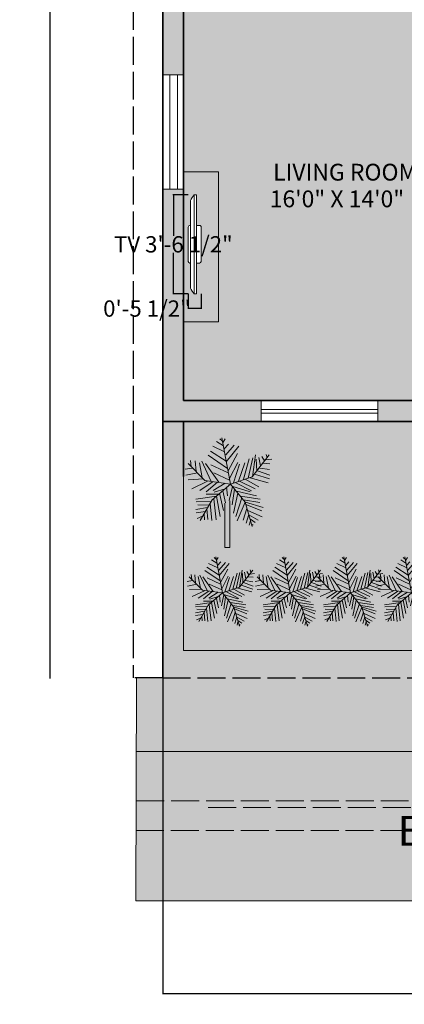
# Model space of a CAD drawing. Units: inches. Extents: x 1316 to 1777, y 813 to 1650.
# Tile 1 of 22: x 1316 to 1481, y 813 to 1237. Entities that reach past the tile are written whole.
import ezdxf

# ---------------------------------------------------------------- set-up
doc = ezdxf.new("R2010")
doc.units = ezdxf.units.IN
doc.header["$MEASUREMENT"] = 0
doc.linetypes.add('ACAD_ISO02W100', pattern=[15, 12, -3])
for name, color, linetype, lineweight in [('A-ANNO-DIMS', 2, 'Continuous', 18), ('A-AREA-IDEN', 7, 'Continuous', 18), ('A-EQPM', 8, 'Continuous', 18), ('A-FURN-PATT', 23, 'Continuous', 13), ('A-WALL-PATT', 250, 'Continuous', 13), ('C-PROP', 8, 'ACAD_ISO02W100', 25), ('C-ROAD', 8, 'Continuous', 18), ('C-ROAD-MARK', 9, 'ACAD_ISO02W100', 13), ('C-ROAD-PATT', 251, 'Continuous', 13), ('furniture', 23, 'Continuous', 18), ('greenary', 106, 'Continuous', 13), ('L-HRDS', 8, 'Continuous', 18), ('L-HRDS-PATT', 252, 'Continuous', 13), ('L-PLNT-PATT', 74, 'Continuous', 13), ('text', 7, 'Continuous', 18), ('walls', 250, 'Continuous', 35), ('windows', 141, 'Continuous', 18)]:
    doc.layers.add(name, color=color, linetype=linetype, lineweight=lineweight)
doc.layers.add('A-FLOR-PATT', color=254, linetype='Continuous', lineweight=13, true_color=0xfeeab9)
doc.styles.get("Standard").update_dxf_attribs({"font": 'arial.ttf'})
doc.dimstyles.get("Standard").update_dxf_attribs({"dimtxt": 7, "dimasz": 0.18, "dimexe": 0.18, "dimexo": 0.0625, "dimgap": 0.09, "dimtad": 0, "dimtih": 1, "dimtoh": 1, "dimzin": 0, "dimdsep": 46, "dimlunit": 3, "dimtxsty": 'Standard', "dimcen": 0.09, "dimadec": 0, "dimazin": 0, "dimtfac": 1, "dimtofl": 0, "dimtmove": 0, "dimatfit": 3, "dimfxl": 1, "dimtolj": 1, "dimtzin": 0, "dimarcsym": 0})

# ---------------------------------------------------------------- blocks, each defined once
blk = doc.blocks.new('PLASMA-LARGE')
at = {"layer": 'furniture'}
for p, q in [((-7.26, 0), (7.26, 0)), ((-21, -2.5), (21, -2.5)), ((-21, -2.5), (-21, -3.5)), ((-21, -3.5), (21, -3.5)), ((-18.61, -1), (18.61, -1)), ((-8, -1), (-8, -0.74)), ((-8, -3.5), (-8, -4.76)), ((8, -1), (8, -0.74)), ((8, -3.5), (8, -4.76)), ((21, -2.5), (21, -3.5)), ((-7.26, -5.5), (7.26, -5.5))]:
    blk.add_line(p, q, dxfattribs=at)
for centre, radius, start, end in [((-7.26, -0.74), 0.744, 90, 180), ((7.26, -0.74), 0.744, 0, 90), ((-13.97, -11.05), 11.07, 114.7602, 129.4175), ((13.97, -11.05), 11.07, 50.5825, 65.2398), ((-7.26, -4.76), 0.744, 180, 270), ((7.26, -4.76), 0.744, 270, 0)]:
    blk.add_arc(centre, radius, start, end, dxfattribs=at)
blk = doc.blocks.new('*U13')
for p, q in [((-8.737, 47.138), (-17.069, 52.711)), ((-10.186, 53.64), (-13.084, 55.962)), ((0, 0), (-10.5, 57)), ((-9.099, 51.782), (-6.563, 55.962)), ((-7.65, 43.423), (-2.578, 49.46)), ((-5.114, 28.097), (-24.676, 40.636)), ((-7.288, 39.707), (-21.778, 46.673)), ((-5.839, 35.992), (4.667, 48.067)), ((-5.114, 27.632), (10.463, 46.673)), ((-2.941, 16.486), (8.652, 37.85)), ((-31.5, 4.5), (-52.5, 25.5)), ((-48.585, 21.131), (-49.309, 29.026)), ((-43.513, 28.561), (-42.427, 15.558)), ((-38.442, 26.239), (-34.819, 7.663)), ((-35.544, 28.097), (-24.314, 3.947)), ((-14.533, 2.09), (-30.834, 25.31)), ((-3.665, 19.273), (-27.574, 35.527)), ((-1.129, 6.734), (9.014, 26.704)), ((3.942, 1.625), (11.187, 24.381)), ((10.101, 3.483), (17.708, 26.239)), ((16.259, 5.805), (23.142, 31.348)), ((22.055, 7.198), (27.489, 32.277)), ((27, 9), (48, 36)), ((27.127, 9.056), (31.112, 35.992)), ((31.836, 30.883), (32.561, 16.486)), ((35.096, 32.741), (37.27, 22.524)), ((38.719, 34.134), (41.979, 28.561)), ((40.53, 25.775), (48.862, 24.846)), ((43.791, 29.954), (51.036, 30.883)), ((44.153, 36.456), (45.239, 32.741)), ((-47.498, 19.737), (-55.83, 18.344)), ((-40.615, 13.7), (-55.105, 10.913)), ((-24.314, 23.917), (-2.941, 13.7)), ((-20.691, 13.7), (-1.129, 4.876)), ((29.662, 12.307), (48.137, 6.269)), ((33.285, 16.486), (48.862, 10.913)), ((36.183, 19.737), (48.137, 17.88)), ((-33.37, 6.269), (-52.207, 5.34)), ((-28.299, 3.483), (-47.86, -5.805)), ((-21.416, 3.018), (-38.079, -8.128)), ((0, 0), (-31.5, 4.5)), ((-15.982, 2.09), (-30.11, -9.521)), ((0, 0), (-22.5, -19.5)), ((-6.563, 1.161), (-21.416, -8.128)), ((0, 0), (27, 9)), ((0, 0), (18, -22.5)), ((6.478, 1.625), (26.04, -8.592)), ((11.187, 3.483), (30.749, -5.805)), ((18.07, 5.805), (35.096, -3.483)), ((24.229, 7.663), (46.688, 1.625)), ((-6.563, -5.805), (-19.967, -9.985)), ((-13.446, -11.378), (-8.737, -32.741)), ((-9.461, -8.592), (-6.201, -23.453)), ((-4.752, -3.483), (-3.665, -14.629)), ((2.493, -3.019), (-1.491, -20.202)), ((1.769, -2.555), (24.229, -9.521)), ((5.029, -6.27), (2.131, -25.775)), ((9.014, -11.378), (3.58, -35.992)), ((7.565, -9.056), (32.198, -14.629)), ((-17.431, -15.094), (-42.789, -18.809)), ((-24.314, -21.596), (-42.427, -22.06)), ((-22.5, -19.5), (-37.5, -45)), ((-15.257, -12.772), (-30.11, -12.772)), ((-25.038, -23.918), (-22.865, -45.281)), ((-20.691, -18.345), (-17.793, -44.352)), ((-17.069, -15.094), (-12.721, -40.172)), ((14.085, -16.951), (6.478, -40.172)), ((18.07, -22.524), (8.289, -45.745)), ((12.274, -15.094), (36.907, -18.809)), ((16.259, -19.738), (36.183, -22.989)), ((18, -22.5), (27, -52.5)), ((18.433, -22.524), (40.53, -29.026)), ((-28.299, -29.026), (-42.789, -31.348)), ((-30.834, -34.135), (-42.427, -35.528)), ((-26.849, -26.24), (-40.253, -25.775)), ((-29.023, -30.884), (-27.936, -43.887)), ((20.244, -30.419), (15.897, -44.816)), ((19.157, -25.311), (38.719, -33.206)), ((21.331, -32.741), (39.081, -40.636)), ((-34.457, -39.708), (-40.978, -42.494)), ((-32.646, -36.921), (-31.921, -44.352)), ((22.78, -37.85), (19.519, -48.532)), ((22.78, -38.314), (34.372, -44.816)), ((24.591, -45.745), (23.142, -50.854)), ((24.591, -43.423), (30.749, -47.603)), ((26.764, -49.925), (28.213, -50.854))]:
    blk.add_line(p, q)
blk = doc.blocks.new('*D23')
at = {"layer": 'A-ANNO-DIMS', "color": 0, "lineweight": -2, "transparency": 16777216}
for p, q in [((1328.47, 1604.17), (1328.87, 1604.17)), ((1328.69, 1603.99), (1328.69, 1282.59)), ((1328.69, 953.87), (1328.69, 1275.27)), ((1328.47, 953.69), (1328.87, 953.69))]:
    blk.add_line(p, q, dxfattribs=at)
at = {"layer": 'A-ANNO-DIMS', "color": 0, "transparency": 16777216}
for points in [[(1328.66, 1603.99), (1328.72, 1603.99), (1328.69, 1604.17)], [(1328.66, 953.87), (1328.72, 953.87), (1328.69, 953.69)]]:
    blk.add_solid(points, dxfattribs=at)
at = {"layer": 'Defpoints', "color": 0, "transparency": 16777216}
for p in [(1328.4, 1604.17), (1328.4, 953.69), (1328.69, 953.69)]:
    blk.add_point(p, dxfattribs=at)
at = {"layer": 'A-ANNO-DIMS', "color": 0, "transparency": 16777216, "insert": (1328.69, 1278.93), "char_height": 7, "width": 24.3281, "attachment_point": 5}
blk.add_mtext('\\A1;47\'-0"', dxfattribs=at)
blk = doc.blocks.new('*D46')
at = {"layer": 'A-ANNO-DIMS', "color": 0, "lineweight": -2, "transparency": 16777216}
for p, q in [((1387.95, 1161.24), (1381.46, 1161.24)), ((1381.64, 1161.06), (1381.64, 1143.71)), ((1381.64, 1118.95), (1381.64, 1136.29)), ((1387.95, 1118.77), (1381.46, 1118.77))]:
    blk.add_line(p, q, dxfattribs=at)
at = {"layer": 'A-ANNO-DIMS', "color": 0, "transparency": 16777216}
for points in [[(1381.61, 1161.06), (1381.67, 1161.06), (1381.64, 1161.24)], [(1381.61, 1118.95), (1381.67, 1118.95), (1381.64, 1118.77)]]:
    blk.add_solid(points, dxfattribs=at)
at = {"layer": 'Defpoints', "color": 0, "transparency": 16777216}
for p in [(1381.64, 1161.24), (1388.01, 1161.24), (1388.01, 1118.77)]:
    blk.add_point(p, dxfattribs=at)
at = {"layer": 'A-ANNO-DIMS', "color": 0, "transparency": 16777216, "insert": (1381.64, 1140), "char_height": 7, "attachment_point": 5}
blk.add_mtext('\\A1;TV 3\'-6 1/2"', dxfattribs=at)
blk = doc.blocks.new('*D47')
at = {"layer": 'A-ANNO-DIMS', "color": 0, "lineweight": -2, "transparency": 16777216}
for p, q in [((1388.01, 1118.7), (1388.01, 1112.21)), ((1393.58, 1118.7), (1393.58, 1112.21)), ((1388.01, 1112.39), (1387.83, 1112.39)), ((1393.4, 1112.39), (1388.19, 1112.39))]:
    blk.add_line(p, q, dxfattribs=at)
at = {"layer": 'A-ANNO-DIMS', "color": 0, "transparency": 16777216}
for points in [[(1388.19, 1112.42), (1388.19, 1112.36), (1388.01, 1112.39)], [(1393.4, 1112.42), (1393.4, 1112.36), (1393.58, 1112.39)]]:
    blk.add_solid(points, dxfattribs=at)
at = {"layer": 'Defpoints', "color": 0, "transparency": 16777216}
for p in [(1388.01, 1118.77), (1393.58, 1118.77), (1388.01, 1112.39)]:
    blk.add_point(p, dxfattribs=at)
at = {"layer": 'A-ANNO-DIMS', "color": 0, "transparency": 16777216, "insert": (1370.29, 1112.39), "char_height": 7, "attachment_point": 5}
blk.add_mtext('\\A1;0\'-5 1/2"', dxfattribs=at)
blk = doc.blocks.new('*D50')
at = {"layer": 'A-ANNO-DIMS', "color": 0, "lineweight": -2, "transparency": 16777216}
for p, q in [((1377.06, 1063.81), (1377.06, 817.77)), ((1713.17, 1031.11), (1713.17, 817.77)), ((1377.24, 817.95), (1532.95, 817.95)), ((1712.99, 817.95), (1557.29, 817.95))]:
    blk.add_line(p, q, dxfattribs=at)
at = {"layer": 'A-ANNO-DIMS', "color": 0, "transparency": 16777216}
for points in [[(1377.24, 817.98), (1377.24, 817.92), (1377.06, 817.95)], [(1712.99, 817.98), (1712.99, 817.92), (1713.17, 817.95)]]:
    blk.add_solid(points, dxfattribs=at)
at = {"layer": 'Defpoints', "color": 0, "transparency": 16777216}
for p in [(1377.06, 1063.87), (1713.17, 1031.17), (1713.17, 817.95)]:
    blk.add_point(p, dxfattribs=at)
at = {"layer": 'A-ANNO-DIMS', "color": 0, "transparency": 16777216, "insert": (1545.12, 817.95), "char_height": 7, "attachment_point": 5}
blk.add_mtext('\\A1;28\'-0"', dxfattribs=at)

msp = doc.modelspace()

# ---------------------------------------------------------------- hatches: boundary and pattern name
at = {"layer": 'A-FLOR-PATT'}
h = msp.add_hatch(color=256, dxfattribs=at)
h.dxf.hatch_style = 1
h.paths.add_polyline_path([(1567.673, 1281.369), (1651.673, 1281.369), (1651.673, 1365.369), (1597.673, 1365.369), (1597.673, 1429.869), (1570.345, 1429.869), (1570.345, 1471.869), (1510.345, 1471.869), (1510.345, 1429.869), (1444.564, 1429.869), (1444.564, 1322.882), (1444.564, 1300.088), (1510.564, 1300.088), (1510.564, 1295.094), (1510.564, 1240.869), (1386.064, 1240.869), (1386.064, 1171.185), (1400.961, 1171.185), (1400.961, 1106.742), (1386.064, 1106.742), (1386.064, 1072.869), (1510.564, 1072.869), (1510.564, 1040.173), (1541.068, 1040.173, -0.367085), (1572.764, 1069.547), (1572.764, 1069.579), (1574.225, 1069.579), (1574.225, 1040.173), (1616.037, 1040.173), (1616.037, 1086.627), (1616.037, 1103.705), (1613.066, 1105.235), (1616.037, 1106.686), (1616.037, 1123.869), (1567.673, 1123.869)])
h.paths.add_polyline_path([(1508.987, 1198.018), (1511.117, 1198.018), (1511.117, 1200.148), (1532.595, 1200.148), (1532.595, 1198.018), (1534.725, 1198.018), (1534.725, 1176.008), (1530.465, 1176.008), (1530.465, 1176.718), (1513.247, 1176.718), (1513.247, 1176.008), (1508.987, 1176.008)], flags=16)
h.paths.add_polyline_path([(1505.979, 1151.315), (1521.504, 1151.315), (1521.504, 1123.623), (1505.979, 1123.623)], flags=16)
h.paths.add_polyline_path([(1507.734, 1150.101, -1), (1506.932, 1150.101, -1)], flags=0)
h.paths.add_polyline_path([(1512.288, 1138.353), (1512.28, 1138.392), (1512.219, 1138.376)], flags=0)
h.paths.add_polyline_path([(1511.539, 1138.926), (1511.802, 1138.967), (1511.817, 1139.27), (1511.607, 1139.246)], flags=0)
h.paths.add_polyline_path([(1513.745, 1140.234), (1513.68, 1139.885), (1514.014, 1140.045), (1513.855, 1140.308)], flags=0)
h.paths.add_polyline_path([(1513.759, 1139.089), (1514.005, 1139.255), (1513.807, 1139.483), (1513.564, 1139.327)], flags=0)
h.paths.add_polyline_path([(1514.219, 1138.385), (1514.336, 1138.33), (1514.544, 1138.32), (1514.802, 1138.874), (1514.451, 1138.716)], flags=0)
h.paths.add_polyline_path([(1514.577, 1137.439), (1514.573, 1137.4), (1514.699, 1137.4), (1514.696, 1137.402)], flags=0)
h.paths.add_polyline_path([(1512.26, 1136.199), (1512.199, 1136.399), (1512.032, 1136.325), (1512.095, 1136.101), (1512.257, 1136.192)], flags=0)
h.paths.add_polyline_path([(1512.644, 1137.274), (1512.356, 1137.23), (1512.432, 1137.049), (1512.703, 1137.093)], flags=0)
h.paths.add_polyline_path([(1513.049, 1137.593), (1512.979, 1137.8), (1512.843, 1137.757), (1512.887, 1137.556)], flags=0)
h.paths.add_polyline_path([(1513.269, 1138.556), (1513.571, 1137.962), (1513.459, 1136.814), (1513.212, 1137.878), (1513.032, 1138.443)], flags=0)
h.paths.add_polyline_path([(1514.891, 1136.377), (1514.696, 1136.401), (1514.683, 1136.246), (1514.87, 1136.165)], flags=0)
h.paths.add_polyline_path([(1514.142, 1137.293), (1514.047, 1136.743), (1514.27, 1136.751), (1514.328, 1137.265)], flags=0)
h.paths.add_polyline_path([(1515.362, 1138.976), (1515.334, 1138.638), (1515.596, 1138.588), (1515.627, 1138.932)], flags=0)
h.paths.add_polyline_path([(1537.285, 1177.912), (1537.995, 1177.912), (1537.995, 1195.13), (1537.285, 1195.13), (1537.285, 1199.39), (1559.295, 1199.39), (1559.295, 1197.26), (1561.425, 1197.26), (1561.425, 1175.782), (1559.295, 1175.782), (1559.295, 1173.652), (1559.379, 1173.652), (1559.379, 1171.514), (1561.517, 1171.514), (1561.517, 1098.819), (1559.379, 1098.819), (1559.379, 1096.68), (1537.285, 1096.68), (1537.285, 1100.957), (1537.997, 1100.957), (1537.997, 1169.376), (1537.285, 1169.376), (1537.285, 1173.652)], flags=16)
h.paths.add_polyline_path([(1518.623, 1345.565), (1519.133, 1345.48), (1519.133, 1345.485), (1518.623, 1345.567)], flags=16)
h.paths.add_polyline_path([(1518.798, 1374.15), (1519.308, 1374.064), (1519.308, 1374.069), (1518.798, 1374.152)], flags=16)
h.paths.add_polyline_path([(1537.764, 1413.501), (1537.678, 1412.991), (1537.683, 1412.991), (1537.766, 1413.501)], flags=16)
h.paths.add_polyline_path([(1572.905, 1373.821), (1573.927, 1373.975), (1574.027, 1390.309), (1573.007, 1390.475), (1573.007, 1390.475)], flags=16)
h.paths.add_polyline_path([(1572.73, 1345.237), (1573.752, 1345.39), (1573.852, 1361.724), (1572.832, 1361.89), (1572.832, 1361.89)], flags=16)
h.paths.add_polyline_path([(1537.211, 1322.643), (1537.364, 1321.621), (1553.698, 1321.521), (1553.864, 1322.541)], flags=16)
h.paths.add_polyline_path([(1535.908, 1331.328), (1527.214, 1331.382), (1527.664, 1404.885), (1564.416, 1404.66), (1563.966, 1331.157), (1555.273, 1331.21), (1553.947, 1323.051), (1537.134, 1323.154)], flags=16)
h.paths.add_polyline_path([(1536.15, 1336.503), (1536.235, 1337.572), (1536.323, 1338.628), (1536.411, 1339.663), (1536.495, 1340.67), (1536.574, 1341.66), (1536.648, 1342.648), (1536.717, 1343.649), (1536.78, 1344.678), (1536.837, 1345.75), (1536.913, 1347.475), (1536.93, 1348.082), (1536.867, 1346.314), (1536.754, 1344.188), (1536.619, 1342.219), (1536.495, 1340.67), (1536.411, 1339.663), (1536.323, 1338.628), (1536.235, 1337.572), (1536.15, 1336.503), (1536.071, 1335.432), (1536.002, 1334.37), (1535.917, 1332.754), (1535.909, 1332.308), (1535.964, 1333.78), (1536.071, 1335.432)], flags=0)
h.paths.add_polyline_path([(1540.412, 1338.345), (1540.539, 1339.037), (1540.667, 1339.758), (1540.798, 1340.518), (1540.93, 1341.325), (1541.063, 1342.187), (1541.196, 1343.109), (1541.326, 1344.085), (1541.45, 1345.102), (1541.566, 1346.15), (1541.669, 1347.219), (1541.758, 1348.296), (1541.829, 1349.371), (1541.879, 1350.434), (1541.906, 1351.476), (1541.91, 1352.5), (1541.895, 1353.512), (1541.861, 1354.518), (1541.812, 1355.524), (1541.749, 1356.537), (1541.674, 1357.561), (1541.551, 1359.062), (1541.495, 1359.67), (1541.589, 1358.603), (1541.721, 1356.977), (1541.846, 1354.98), (1541.912, 1352.982), (1541.903, 1350.951), (1541.806, 1348.87), (1541.628, 1346.713), (1541.396, 1344.612), (1541.135, 1342.656), (1540.872, 1340.947), (1540.617, 1339.466), (1540.412, 1338.345), (1540.288, 1337.675), (1540.166, 1337.018), (1540.049, 1336.365), (1539.937, 1335.71), (1539.837, 1335.055), (1539.758, 1334.403), (1539.709, 1333.756), (1539.697, 1333.12), (1539.751, 1332.162), (1539.822, 1331.89), (1539.691, 1332.775), (1539.714, 1334.035), (1539.867, 1335.303), (1540.085, 1336.577), (1540.288, 1337.675)], flags=0)
h.paths.add_polyline_path([(1545.599, 1331.584), (1545.601, 1331.617), (1545.614, 1331.689), (1545.737, 1332.197), (1545.767, 1332.332), (1545.84, 1332.681), (1545.925, 1333.114), (1546.016, 1333.614), (1546.108, 1334.164), (1546.196, 1334.748), (1546.276, 1335.349), (1546.342, 1335.952), (1546.388, 1336.539), (1546.412, 1337.098), (1546.414, 1337.632), (1546.395, 1338.145), (1546.359, 1338.645), (1546.306, 1339.137), (1546.24, 1339.627), (1546.161, 1340.121), (1546.073, 1340.625), (1545.888, 1341.63), (1545.718, 1342.621), (1545.547, 1343.945), (1545.432, 1345.534), (1545.404, 1347.402), (1545.418, 1348.013), (1545.411, 1346.957), (1545.425, 1345.988), (1545.463, 1345.105), (1545.521, 1344.301), (1545.596, 1343.566), (1545.683, 1342.892), (1545.778, 1342.27), (1545.877, 1341.691), (1545.977, 1341.145), (1546.133, 1340.297), (1546.327, 1339.075), (1546.434, 1337.615), (1546.377, 1336.279), (1546.246, 1335.079), (1546.032, 1333.665), (1545.84, 1332.681), (1545.767, 1332.332)], flags=0)
h.paths.add_polyline_path([(1551.803, 1337.656), (1551.963, 1338.25), (1552.102, 1338.801), (1552.225, 1339.338), (1552.331, 1339.865), (1552.418, 1340.377), (1552.487, 1340.873), (1552.536, 1341.348), (1552.563, 1341.801), (1552.569, 1342.228), (1552.551, 1342.627), (1552.51, 1342.995), (1552.446, 1343.333), (1552.363, 1343.646), (1552.261, 1343.937), (1552.144, 1344.207), (1552.012, 1344.461), (1551.868, 1344.7), (1551.746, 1344.882), (1550.887, 1346.052), (1550.428, 1347.126), (1550.183, 1348.353), (1550.048, 1349.632), (1549.978, 1351.224), (1549.974, 1353.141), (1549.989, 1353.748), (1549.975, 1352.682), (1549.977, 1351.708), (1549.996, 1350.825), (1550.031, 1350.027), (1550.082, 1349.31), (1550.15, 1348.669), (1550.234, 1348.098), (1550.335, 1347.593), (1550.452, 1347.149), (1550.584, 1346.76), (1550.73, 1346.419), (1550.887, 1346.117), (1551.05, 1345.848), (1551.217, 1345.602), (1551.386, 1345.372), (1551.553, 1345.151), (1552, 1344.537), (1552.454, 1343.495), (1552.591, 1342.266), (1552.509, 1340.905), (1552.246, 1339.367), (1551.925, 1338.101), (1551.619, 1336.984), (1551.406, 1336.2), (1551.01, 1334.699), (1550.877, 1334.155), (1551.264, 1335.677), (1551.619, 1336.984)], flags=0)
h.paths.add_polyline_path([(1558.642, 1348.348), (1558.795, 1348.811), (1558.918, 1349.215), (1559.008, 1349.575), (1559.061, 1349.904), (1559.076, 1350.214), (1559.054, 1350.506), (1559.001, 1350.776), (1558.919, 1351.021), (1558.814, 1351.239), (1558.688, 1351.425), (1558.546, 1351.578), (1558.392, 1351.694), (1558.229, 1351.772), (1558.059, 1351.812), (1557.882, 1351.819), (1557.701, 1351.794), (1557.515, 1351.742), (1557.327, 1351.665), (1557.136, 1351.566), (1556.944, 1351.448), (1556.752, 1351.315), (1556.742, 1351.307), (1556.175, 1350.878), (1555.982, 1350.741), (1555.79, 1350.618), (1555.103, 1350.248), (1554.019, 1350.696), (1553.658, 1351.734), (1553.592, 1352.861), (1553.705, 1354.248), (1553.753, 1354.657), (1553.685, 1354.004), (1553.638, 1353.425), (1553.615, 1352.918), (1553.615, 1352.476), (1553.637, 1352.094), (1553.681, 1351.766), (1553.745, 1351.485), (1553.828, 1351.246), (1553.929, 1351.043), (1554.048, 1350.87), (1554.182, 1350.722), (1554.33, 1350.599), (1554.491, 1350.501), (1554.662, 1350.43), (1554.841, 1350.388), (1555.026, 1350.374), (1555.215, 1350.39), (1555.406, 1350.437), (1555.598, 1350.514), (1555.79, 1350.618), (1555.982, 1350.741), (1556.175, 1350.878), (1556.367, 1351.024), (1556.559, 1351.171), (1556.752, 1351.315), (1556.944, 1351.448), (1557.136, 1351.566), (1557.327, 1351.665), (1558.043, 1351.957), (1558.894, 1351.316), (1559.137, 1350.09), (1558.886, 1349.087), (1558.642, 1348.348), (1558.463, 1347.812), (1558.261, 1347.187), (1558.039, 1346.459), (1557.677, 1345.175), (1557.549, 1344.636), (1557.909, 1346.03), (1558.329, 1347.408)], flags=0)
h.paths.add_polyline_path([(1562.145, 1353.919), (1562.25, 1354.68), (1562.341, 1355.344), (1562.416, 1355.924), (1562.475, 1356.431), (1562.518, 1356.872), (1562.544, 1357.254), (1562.554, 1357.582), (1562.548, 1357.862), (1562.525, 1358.1), (1562.486, 1358.303), (1562.432, 1358.476), (1562.361, 1358.624), (1562.277, 1358.748), (1562.18, 1358.848), (1562.073, 1358.925), (1561.958, 1358.977), (1561.837, 1359.006), (1561.711, 1359.011), (1561.584, 1358.992), (1561.456, 1358.949), (1561.342, 1358.895), (1560.78, 1358.554), (1560.631, 1358.473), (1560.474, 1358.403), (1560.311, 1358.348), (1559.637, 1358.207), (1558.973, 1358.904), (1558.816, 1360.002), (1558.804, 1361.236), (1558.83, 1361.674), (1558.807, 1360.917), (1558.813, 1360.297), (1558.845, 1359.795), (1558.902, 1359.397), (1558.982, 1359.087), (1559.082, 1358.849), (1559.2, 1358.666), (1559.334, 1358.525), (1559.482, 1358.421), (1559.639, 1358.351), (1559.804, 1358.311), (1559.973, 1358.3), (1560.143, 1358.313), (1560.311, 1358.348), (1560.474, 1358.403), (1560.631, 1358.473), (1560.78, 1358.554), (1560.923, 1358.641), (1561.061, 1358.729), (1561.196, 1358.813), (1561.382, 1358.92), (1561.342, 1358.895), (1561.972, 1359.194), (1562.536, 1358.367), (1562.56, 1357.311), (1562.455, 1356.226), (1562.323, 1355.206), (1562.145, 1353.919), (1562.026, 1353.049), (1561.815, 1351.457), (1561.752, 1350.933), (1561.948, 1352.479)], flags=0)
h.paths.add_polyline_path([(1572.764, 1069.547, 0.367085), (1541.068, 1040.173), (1572.764, 1040.173)], flags=17)
h.paths.add_polyline_path([(1572.764, 1040.173), (1541.068, 1040.173, 0.0299535), (1540.829, 1036.182), (1540.829, 1031.173), (1574.225, 1031.173), (1574.225, 1036.182), (1572.764, 1036.182)])
at = {"layer": 'A-FURN-PATT'}
h = msp.add_hatch(color=256, dxfattribs=at)
h.dxf.hatch_style = 1
h.paths.add_polyline_path([(1400.961, 1171.185), (1386.064, 1171.185), (1386.064, 1106.742), (1400.961, 1106.742)])
h.paths.add_polyline_path([(1391.554, 1118.766), (1390.543, 1118.766, -0.0640419), (1389.026, 1121.185), (1389.026, 1131.913), (1388.767, 1131.913, -0.4142136), (1388.015, 1132.665), (1388.015, 1147.341, -0.4142136), (1388.767, 1148.093), (1389.026, 1148.093), (1389.026, 1158.821, -0.0640419), (1390.543, 1161.24), (1391.554, 1161.24), (1391.554, 1148.093), (1392.824, 1148.093, -0.4142136), (1393.577, 1147.341), (1393.577, 1132.665, -0.4142136), (1392.824, 1131.913), (1391.554, 1131.913)], flags=16)
at = {"layer": 'A-WALL-PATT'}
h = msp.add_hatch(color=256, dxfattribs=at)
h.dxf.hatch_style = 1
h.paths.add_polyline_path([(1713.173, 1281.369), (1656.173, 1281.369), (1656.173, 1298.258), (1651.673, 1298.258), (1651.673, 1281.369), (1567.673, 1281.369), (1567.673, 1266.995), (1572.173, 1266.995), (1572.173, 1276.869), (1704.173, 1276.869), (1704.173, 1132.869), (1608.64, 1132.869), (1608.64, 1123.869), (1704.173, 1123.869), (1704.173, 1040.173), (1652.869, 1040.173), (1652.869, 1031.173), (1713.173, 1031.173), (1713.173, 1040.173)])
h.paths.add_polyline_path([(1572.173, 1237.955), (1567.673, 1237.955), (1567.673, 1123.869), (1583.146, 1123.869), (1583.146, 1132.869), (1572.173, 1132.869)], flags=17)
h.paths.add_polyline_path([(1510.345, 1566.369), (1524.171, 1566.369), (1524.171, 1571.985), (1524.171, 1575.369), (1445.955, 1575.369), (1445.955, 1566.369), (1505.845, 1566.369), (1505.845, 1469.591), (1510.345, 1469.591), (1510.345, 1471.869), (1529.081, 1471.869), (1529.081, 1476.369), (1510.345, 1476.369)])
h.paths.add_polyline_path([(1609.722, 1575.369), (1545.119, 1575.369), (1545.119, 1566.369), (1570.345, 1566.369), (1570.345, 1476.369), (1562.477, 1476.369), (1562.477, 1471.869), (1570.345, 1471.869), (1570.345, 1469.591), (1574.845, 1469.591), (1574.845, 1566.369), (1609.722, 1566.369)])
h.paths.add_polyline_path([(1713.173, 1575.369), (1655.233, 1575.369), (1655.233, 1566.369), (1704.173, 1566.369), (1704.173, 1434.369), (1574.845, 1434.369), (1574.845, 1440.551), (1574.701, 1440.551), (1570.345, 1440.551), (1570.345, 1429.869), (1597.673, 1429.869), (1597.673, 1408.281), (1602.173, 1408.281), (1602.173, 1429.869), (1704.173, 1429.869), (1704.173, 1410.704), (1707.375, 1410.704), (1713.173, 1410.704)])
h.paths.add_polyline_path([(1713.173, 1383.676), (1704.173, 1383.676), (1704.173, 1369.869), (1602.173, 1369.869), (1602.173, 1379.241), (1597.673, 1379.241), (1597.673, 1365.369), (1713.173, 1365.369)])
h.paths.add_polyline_path([(1444.564, 1429.869), (1510.345, 1429.869), (1510.345, 1440.551), (1505.845, 1440.551), (1505.845, 1434.369), (1386.064, 1434.369), (1386.064, 1566.369), (1400.445, 1566.369), (1400.445, 1575.369), (1377.064, 1575.369), (1377.064, 1412.813), (1380.509, 1412.813), (1386.064, 1412.813), (1386.064, 1429.869), (1440.064, 1429.869), (1440.064, 1401.229), (1444.564, 1401.229)])
h.paths.add_polyline_path([(1444.564, 1372.189), (1440.064, 1372.189), (1440.064, 1369.869), (1386.064, 1369.869), (1386.064, 1378.758), (1377.064, 1378.758), (1377.064, 1349.201), (1381.118, 1349.201), (1386.064, 1349.201), (1386.064, 1365.369), (1440.064, 1365.369), (1440.064, 1322.882), (1444.564, 1322.882)])
h.paths.add_polyline_path([(1510.564, 1295.094), (1506.064, 1295.094), (1506.064, 1245.369), (1386.064, 1245.369), (1386.064, 1272.582), (1377.064, 1272.582), (1377.064, 1212.905), (1380.1, 1212.905), (1386.064, 1212.905), (1386.064, 1240.869), (1510.564, 1240.869)])
h.paths.add_polyline_path([(1386.064, 1163.761), (1377.064, 1163.761), (1377.064, 1063.869), (1419.363, 1063.869), (1419.363, 1072.869), (1386.064, 1072.869)])
h.paths.add_polyline_path([(1510.564, 1072.869), (1469.381, 1072.869), (1469.381, 1063.869), (1501.564, 1063.869), (1501.564, 1033.023), (1501.564, 1031.173), (1540.829, 1031.173), (1540.829, 1036.182, -0.0299535), (1541.068, 1040.173), (1510.564, 1040.173)])
h.paths.add_polyline_path([(1607.369, 1040.173), (1574.225, 1040.173), (1574.225, 1036.182), (1574.225, 1031.173), (1607.369, 1031.173)], flags=17)
h.paths.add_polyline_path([(1637.054, 1040.173), (1624.706, 1040.173), (1624.706, 1031.173), (1637.054, 1031.173)], flags=17)
at = {"layer": 'C-ROAD-PATT'}
h = msp.add_hatch(color=256, dxfattribs=at)
h.dxf.hatch_style = 1
h.paths.add_polyline_path([(1724.399, 922.018), (1494.583, 922.018), (1365.735, 922.018), (1365.534, 857.849), (1713.173, 857.849), (1724.399, 857.849)])
h = msp.add_hatch(color=256, dxfattribs=at)
h.dxf.hatch_style = 1
h.paths.add_polyline_path([(1724.399, 875.958), (1724.399, 915.982), (1365.716, 915.982), (1365.591, 875.958)])
at = {"layer": 'L-HRDS-PATT'}
h = msp.add_hatch(color=256, dxfattribs=at)
h.dxf.hatch_style = 1
h.paths.add_polyline_path([(1492.539, 953.689), (1377.064, 953.689), (1365.834, 953.689), (1365.735, 922.018), (1492.539, 922.018)])
h.paths.add_polyline_path([(1724.399, 953.689), (1713.173, 953.689), (1606.561, 953.689), (1606.561, 922.018), (1724.399, 922.018)])
h.paths.add_polyline_path([(1667.146, 959.936), (1596.428, 959.936), (1596.428, 953.689), (1604.517, 953.689), (1604.517, 955.706), (1606.561, 955.706), (1606.561, 953.689), (1667.146, 953.689)])
h.paths.add_polyline_path([(1704.173, 1123.869), (1685.903, 1123.869), (1685.903, 1062.613), (1672.026, 1062.613), (1668.679, 1062.613), (1668.679, 1040.173), (1704.173, 1040.173)])
h = msp.add_hatch(color=256, dxfattribs=at)
h.dxf.hatch_style = 1
h.paths.add_polyline_path([(1501.564, 965.355), (1386.064, 965.355), (1386.064, 1063.869), (1377.064, 1063.869), (1377.064, 953.689), (1492.539, 953.689), (1492.539, 955.706), (1494.583, 955.706), (1494.583, 953.689), (1501.564, 953.689)])
at = {"layer": 'L-PLNT-PATT'}
h = msp.add_hatch(color=256, dxfattribs=at)
h.dxf.hatch_style = 1
h.paths.add_polyline_path([(1501.564, 1031.173), (1501.564, 1033.023), (1501.564, 1063.869), (1386.064, 1063.869), (1386.064, 965.355), (1501.564, 965.355)])
h.paths.add_polyline_path([(1668.679, 1062.613), (1617.549, 1062.613), (1617.549, 1040.173), (1624.706, 1040.173), (1668.679, 1040.173)])

# ---------------------------------------------------------------- linework, layer by layer
at = {"layer": 'C-PROP'}
for p, q in [((1364.399, 1604.173), (1364.399, 953.689)), ((1377.064, 953.689), (1364.399, 953.689)), ((1377.064, 953.689), (1713.173, 953.689))]:
    msp.add_line(p, q, dxfattribs=at)
at = {"layer": 'C-ROAD'}
for p, q in [((1365.834, 953.689), (1365.534, 857.849)), ((1365.534, 922.018), (1494.583, 922.018)), ((1365.534, 857.849), (1713.173, 857.849))]:
    msp.add_line(p, q, dxfattribs=at)
at = {"layer": 'C-ROAD-MARK'}
for p, q in [((1365.669, 900.851), (1724.399, 900.851)), ((1396.572, 897.973), (1657.977, 897.973)), ((1365.629, 888.109), (1724.399, 888.109))]:
    msp.add_line(p, q, dxfattribs=at)
at = {"layer": 'furniture'}
for p, q in [((1386.064, 1171.185), (1400.961, 1171.185)), ((1386.064, 1171.185), (1386.064, 1106.742)), ((1400.961, 1171.185), (1400.961, 1106.742)), ((1400.961, 1106.742), (1386.064, 1106.742))]:
    msp.add_line(p, q, dxfattribs=at)
at = {"layer": 'greenary'}
for p, q in [((1403.732, 1028.808), (1403.732, 1009.652)), ((1405.944, 1009.76), (1405.944, 1029.803)), ((1403.732, 1009.652), (1405.944, 1009.76))]:
    msp.add_line(p, q, dxfattribs=at)
at = {"layer": 'L-HRDS'}
for p, q in [((1386.064, 1063.869), (1386.064, 965.355)), ((1386.064, 965.355), (1501.564, 965.355))]:
    msp.add_line(p, q, dxfattribs=at)
at = {"layer": 'walls'}
for p, q in [((1377.064, 1575.369), (1377.064, 953.689)), ((1386.064, 1240.869), (1386.064, 1072.869)), ((1386.064, 1072.869), (1510.564, 1072.869)), ((1377.064, 1063.869), (1501.564, 1063.869)), ((1386.064, 1063.869), (1386.064, 1040.173))]:
    msp.add_line(p, q, dxfattribs=at)
at = {"layer": 'windows'}
for p, q in [((1377.064, 1212.905), (1386.064, 1212.905)), ((1377.064, 1163.761), (1377.064, 1212.905)), ((1377.064, 1212.905), (1380.1, 1212.905)), ((1380.1, 1212.905), (1380.1, 1163.761)), ((1383.37, 1163.761), (1383.37, 1212.905)), ((1386.064, 1212.905), (1386.064, 1163.761)), ((1386.064, 1163.761), (1377.064, 1163.761)), ((1380.1, 1163.761), (1383.37, 1163.761)), ((1419.363, 1072.869), (1419.363, 1063.869)), ((1469.381, 1072.869), (1419.363, 1072.869)), ((1419.363, 1072.869), (1419.363, 1069.072)), ((1469.381, 1063.869), (1469.381, 1072.869)), ((1419.363, 1069.072), (1469.381, 1069.072)), ((1469.381, 1067.411), (1419.363, 1067.411)), ((1469.381, 1069.072), (1469.381, 1067.411)), ((1419.363, 1063.869), (1469.381, 1063.869))]:
    msp.add_line(p, q, dxfattribs=at)

# ---------------------------------------------------------------- block references
at = {"layer": 'A-EQPM', "xscale": 1.011294184530666, "yscale": 1.011294184530666, "zscale": 1.011294184530666, "rotation": 90.00000000000003}
msp.add_blockref('PLASMA-LARGE', (1388.015, 1140.003), dxfattribs=at)
at = {"layer": 'greenary'}
for p, xscale, yscale, zscale in [((1406.169, 1036.977), 0.3471750040413432, 0.3471750040413432, 0.3471750040413432), ((1402.703, 990.151), 0.271325619196482, 0.271325619196482, 0.271325619196482), ((1431.864, 990.151), 0.271325619196482, 0.271325619196482, 0.271325619196482), ((1457.734, 990.151), 0.271325619196482, 0.271325619196482, 0.271325619196482), ((1483.897, 990.151), 0.271325619196482, 0.271325619196482, 0.271325619196482)]:
    msp.add_blockref('*U13', p, dxfattribs=dict(at, xscale=xscale, yscale=yscale, zscale=zscale))

# ---------------------------------------------------------------- texts
at = {"layer": 'A-AREA-IDEN'}
for s, p in [('LIVING ROOM', (1424.507, 1167.396)), ('16\'0" X 14\'0"', (1423.028, 1155.927))]:
    msp.add_text(s, height=7.22716, dxfattribs=at).set_placement(p)
at = {"layer": 'text'}
msp.add_text('E A S T  R O A D', height=12.82247, dxfattribs=at).set_placement((1477.977, 881.478))

# ---------------------------------------------------------------- dimensions: what is measured, and where the dimension line sits
at = {"layer": 'A-ANNO-DIMS'}
for base, p1, p2, text, override, picture, middle in [((1328.686, 953.689), (1328.404, 1604.173), (1328.404, 953.689), '47\'-0"', {"dimclrd": 0, "dimclre": 0, "dimclrt": 0}, '*D23', (1328.686, 1278.931)), ((1381.644, 1161.24), (1388.015, 1118.766), (1388.015, 1161.24), 'TV <>', {"dimdec": 1, "dimlfac": 1, "dimrnd": 0, "dimzin": 1, "dimdsep": 46, "dimlunit": 4, "dimfrac": 2}, '*D46', (1381.644, 1140.003))]:
    dim = msp.add_linear_dim(base=base, p1=p1, p2=p2, angle=90, text=text, dimstyle='Standard', override=override, dxfattribs=at)
    dim.commit()
    dim.dimension.update_dxf_attribs({"geometry": picture, "text_midpoint": middle})
dim = msp.add_linear_dim(base=(1388.015, 1112.395), p1=(1393.577, 1118.766), p2=(1388.015, 1118.766), angle=180, dimstyle='Standard', override={"dimdec": 1, "dimlfac": 1, "dimrnd": 0, "dimzin": 1, "dimdsep": 46, "dimlunit": 4, "dimfrac": 2}, dxfattribs=at)
dim.commit()
dim.dimension.update_dxf_attribs({"geometry": '*D47', "text_midpoint": (1370.285, 1112.395)})
dim = msp.add_linear_dim(base=(1713.173, 817.949), p1=(1377.064, 1063.869), p2=(1713.173, 1031.173), dimstyle='Standard', override={"dimdec": 1, "dimlfac": 1, "dimrnd": 0, "dimzin": 1, "dimdsep": 46, "dimlunit": 4, "dimfrac": 2}, dxfattribs=at)
dim.commit()
dim.dimension.update_dxf_attribs({"geometry": '*D50', "text_midpoint": (1545.119, 817.949)})

doc.saveas('drawing.dxf')
